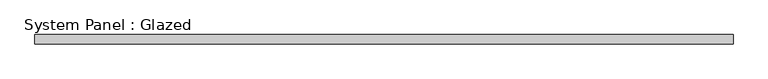
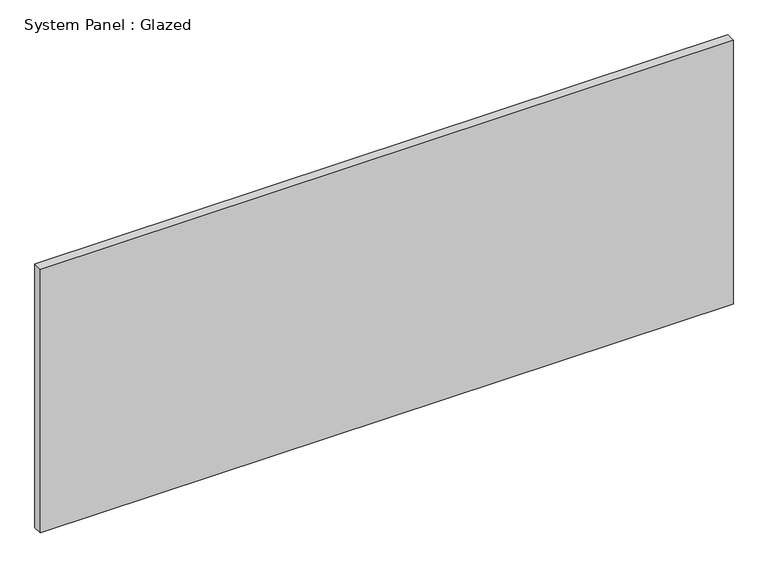
"""IFC4 building model written with IfcOpenShell, lengths in millimetres: plate geometry, System Panel : Glazed."""

from ifc_helpers import new_model, si_unit, origin, origin_with_axes, place, context, project, spatial, polyline, outline, extrude, source, transform, mapped, element, save


def system_panel_glazed_6338a664(model_context):
    return source(origin(), model_context, "Body", "SweptSolid", [
        extrude(outline(polyline([(915.0000002, 24.5), (-915.0000002, 24.5), (-915.0000002, 49.5), (915.0000002, 49.5), (915.0000002, 24.5)])), origin_with_axes(), (0.0, 0.0, 1.0), 736.6),
    ])


if __name__ == "__main__":
    model = new_model("IFC4")
    model_context = context("Model", 3, world=origin())
    ifc_project = project(units=[si_unit("LENGTHUNIT", "METRE", prefix="MILLI")], contexts=[model_context])
    site = spatial("IfcSite", under=ifc_project)
    building = spatial("IfcBuilding", under=site)
    placement = place(None, origin())
    system_panel_glazed_shape = system_panel_glazed_6338a664(model_context)
    element("IfcPlate", 1, ObjectType="System Panel : Glazed", at=placement, inside=building, context=model_context, shape_type="MappedRepresentation", body=[
        mapped(system_panel_glazed_shape, transform((0.0, 0.0, 0.0), x_axis=(1.0, 0.0, 0.0), y_axis=(0.0, 1.0, 0.0), z_axis=(0.0, 0.0, 1.0))),
    ])
    save(model, "model.ifc")

# Revit data of these elements
# Type "System Panel : Glazed"
#   Keynote = "H11"
#   Construction Type Id = "GSP4R"
#   Analytic Construction = "1/8 in Pilkington single glazing"
#   Visual Light Transmittance = 0.9
#   Solar Heat Gain Coefficient = 0.86
#   Heat Transfer Coefficient (U) = 6.7069 W/(m²·K)
#   Define Thermal Properties by = 1
# Element 1 (IfcPlate, "System Panel : Glazed")
#   Materials on its faces: "Glass"
# Materials
#   "Glass": class "Glass", colour RGB 0 128 192, transparency 0.9, Description = "Soda Lime Glass", Cost = 0
